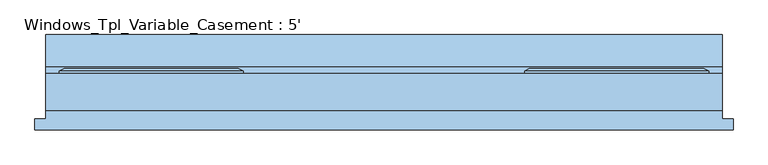
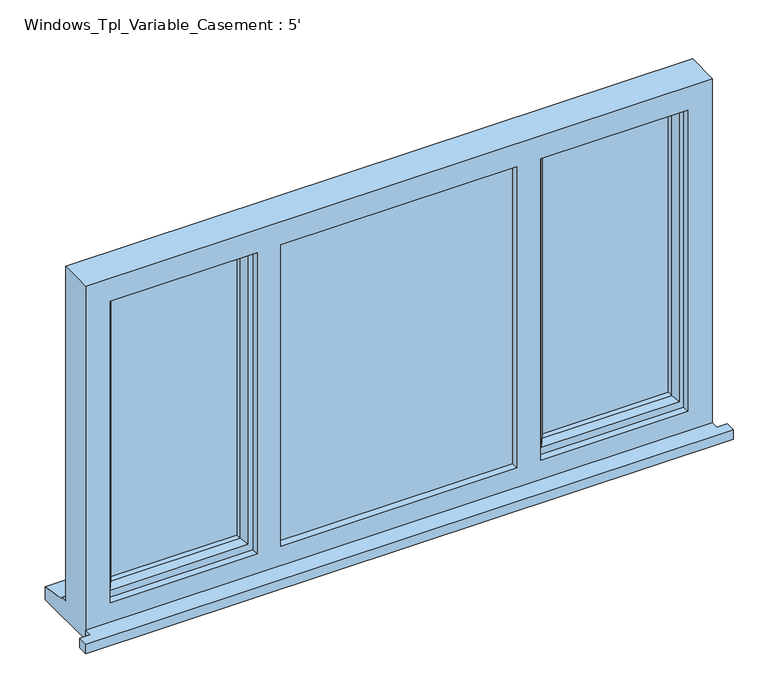
"""IFC4 building model written with IfcOpenShell, lengths in millimetres: window geometry, Windows_Tpl_Variable_Casement : 5'."""

from ifc_helpers import new_model, si_unit, frame, origin, place, context, project, spatial, polyline, outline, extrude, faceted_brep, source, transform, mapped, element, save


def windows_tpl_variable_casement_5_ffad3fa3(model_context):
    return source(origin(), model_context, "Body", "SolidModel", [
        extrude(outline(polyline([(-1234.0, -92.7434322), (-1234.0, -67.7434322), (-1209.0, -67.7434322), (-1209.0, -48.3434322), (315.0, -48.3434322), (315.0, -67.7434322), (340.0, -67.7434322), (340.0, -92.7434322), (-1234.0, -92.7434322)])), frame((0.0, 0.0, 1200.0), z_axis=(0.0, 0.0, 1.0), x_axis=(1.0, 0.0, 0.0)), (0.0, 0.0, 1.0), 25.0),
        faceted_brep([(-130.0, 34.6565678, 2080.0), (-130.0, 40.4300705, 2080.0), (-130.0, 40.4300705, 1253.0), (-130.0, 34.6565678, 1253.0), (-120.0, -30.3434322, 2070.0), (-120.0, 34.6565678, 2070.0), (-120.0, 34.6565678, 1263.0), (-120.0, -30.3434322, 1263.0), (-80.0, -15.8505323, 2030.0), (-90.1480377, -30.3434322, 2040.1480377), (-90.1480377, -30.3434322, 1292.8519623), (-80.0, -15.8505323, 1303.0), (-80.0, -1.3434322, 2030.0), (-80.0, -1.3434322, 1303.0), (-90.0, 22.6565678, 2040.0), (-90.0, -1.3434322, 2040.0), (-90.0, -1.3434322, 1293.0), (-90.0, 22.6565678, 1293.0), (-80.0, 40.4300705, 2030.0), (-80.0, 22.6565678, 2030.0), (-80.0, 22.6565678, 1303.0), (-80.0, 40.4300705, 1303.0), (-97.4457548, 46.2035732, 2047.4457548), (-97.4457548, 46.2035732, 1285.5542452), (-119.2153903, 46.2035732, 2069.2153903), (-119.2153903, 46.2035732, 1263.7846097), (285.0, 40.4300705, 1253.0), (285.0, 34.6565678, 1253.0), (275.0, 34.6565678, 1263.0), (275.0, -30.3434322, 1263.0), (245.1480377, -30.3434322, 1292.8519623), (235.0, -15.8505323, 1303.0), (235.0, -1.3434322, 1303.0), (245.0, -1.3434322, 1293.0), (245.0, 22.6565678, 1293.0), (235.0, 22.6565678, 1303.0), (235.0, 40.4300705, 1303.0), (252.4457548, 46.2035732, 1285.5542452), (274.2153903, 46.2035732, 1263.7846097), (285.0, 40.4300705, 2080.0), (285.0, 34.6565678, 2080.0), (275.0, 34.6565678, 2070.0), (275.0, -30.3434322, 2070.0), (245.1480377, -30.3434322, 2040.1480377), (235.0, -15.8505323, 2030.0), (235.0, -1.3434322, 2030.0), (245.0, -1.3434322, 2040.0), (245.0, 22.6565678, 2040.0), (235.0, 22.6565678, 2030.0), (235.0, 40.4300705, 2030.0), (252.4457548, 46.2035732, 2047.4457548), (274.2153903, 46.2035732, 2069.2153903)], [[[0, 1, 2, 3]], [[4, 5, 6, 7]], [[8, 9, 10, 11]], [[12, 8, 11, 13]], [[14, 15, 16, 17]], [[18, 19, 20, 21]], [[22, 18, 21, 23]], [[1, 24, 25, 2]], [[3, 2, 26, 27]], [[7, 6, 28, 29]], [[11, 10, 30, 31]], [[13, 11, 31, 32]], [[17, 16, 33, 34]], [[21, 20, 35, 36]], [[23, 21, 36, 37]], [[2, 25, 38, 26]], [[27, 26, 39, 40]], [[29, 28, 41, 42]], [[31, 30, 43, 44]], [[32, 31, 44, 45]], [[34, 33, 46, 47]], [[36, 35, 48, 49]], [[37, 36, 49, 50]], [[26, 38, 51, 39]], [[40, 39, 1, 0]], [[3, 27, 40, 0], [5, 41, 28, 6]], [[42, 41, 5, 4]], [[7, 29, 42, 4], [9, 43, 30, 10]], [[44, 43, 9, 8]], [[45, 44, 8, 12]], [[15, 46, 33, 16], [13, 32, 45, 12]], [[47, 46, 15, 14]], [[17, 34, 47, 14], [19, 48, 35, 20]], [[49, 48, 19, 18]], [[50, 49, 18, 22]], [[24, 51, 38, 25], [23, 37, 50, 22]], [[39, 51, 24, 1]]]),
        faceted_brep([(-764.0, 34.6565678, 2080.0), (-764.0, 40.4300705, 2080.0), (-1179.0, 40.4300705, 2080.0), (-1179.0, 34.6565678, 2080.0), (-774.0, -30.3434322, 2070.0), (-774.0, 34.6565678, 2070.0), (-1169.0, 34.6565678, 2070.0), (-1169.0, -30.3434322, 2070.0), (-814.0, -15.8505323, 2030.0), (-803.8519623, -30.3434322, 2040.1480377), (-1139.1480377, -30.3434322, 2040.1480377), (-1129.0, -15.8505323, 2030.0), (-814.0, -1.3434322, 2030.0), (-1129.0, -1.3434322, 2030.0), (-804.0, 22.6565678, 2040.0), (-804.0, -1.3434322, 2040.0), (-1139.0, -1.3434322, 2040.0), (-1139.0, 22.6565678, 2040.0), (-814.0, 40.4300705, 2030.0), (-814.0, 22.6565678, 2030.0), (-1129.0, 22.6565678, 2030.0), (-1129.0, 40.4300705, 2030.0), (-795.1854344, 46.2035732, 2048.8145656), (-1147.8145656, 46.2035732, 2048.8145656), (-775.6307806, 46.2035732, 2068.3692194), (-1167.3692194, 46.2035732, 2068.3692194), (-1179.0, 40.4300705, 1253.0), (-1179.0, 34.6565678, 1253.0), (-1169.0, 34.6565678, 1263.0), (-1169.0, -30.3434322, 1263.0), (-1139.1480377, -30.3434322, 1292.8519623), (-1129.0, -15.8505323, 1303.0), (-1129.0, -1.3434322, 1303.0), (-1139.0, -1.3434322, 1293.0), (-1139.0, 22.6565678, 1293.0), (-1129.0, 22.6565678, 1303.0), (-1129.0, 40.4300705, 1303.0), (-1147.8145656, 46.2035732, 1284.1854344), (-1167.3692194, 46.2035732, 1264.6307806), (-764.0, 40.4300705, 1253.0), (-764.0, 34.6565678, 1253.0), (-774.0, 34.6565678, 1263.0), (-774.0, -30.3434322, 1263.0), (-803.8519623, -30.3434322, 1292.8519623), (-814.0, -15.8505323, 1303.0), (-814.0, -1.3434322, 1303.0), (-804.0, -1.3434322, 1293.0), (-804.0, 22.6565678, 1293.0), (-814.0, 22.6565678, 1303.0), (-814.0, 40.4300705, 1303.0), (-795.1854344, 46.2035732, 1284.1854344), (-775.6307806, 46.2035732, 1264.6307806)], [[[0, 1, 2, 3]], [[4, 5, 6, 7]], [[8, 9, 10, 11]], [[12, 8, 11, 13]], [[14, 15, 16, 17]], [[18, 19, 20, 21]], [[22, 18, 21, 23]], [[1, 24, 25, 2]], [[3, 2, 26, 27]], [[7, 6, 28, 29]], [[11, 10, 30, 31]], [[13, 11, 31, 32]], [[17, 16, 33, 34]], [[21, 20, 35, 36]], [[23, 21, 36, 37]], [[2, 25, 38, 26]], [[27, 26, 39, 40]], [[0, 3, 27, 40], [41, 28, 6, 5]], [[29, 28, 41, 42]], [[4, 7, 29, 42], [43, 30, 10, 9]], [[31, 30, 43, 44]], [[32, 31, 44, 45]], [[46, 33, 16, 15], [12, 13, 32, 45]], [[34, 33, 46, 47]], [[14, 17, 34, 47], [48, 35, 20, 19]], [[36, 35, 48, 49]], [[37, 36, 49, 50]], [[51, 38, 25, 24], [22, 23, 37, 50]], [[26, 38, 51, 39]], [[40, 39, 1, 0]], [[42, 41, 5, 4]], [[44, 43, 9, 8]], [[45, 44, 8, 12]], [[47, 46, 15, 14]], [[49, 48, 19, 18]], [[50, 49, 18, 22]], [[39, 51, 24, 1]]]),
        faceted_brep([(315.0, -48.3434322, 2110.0), (-1209.0, -48.3434322, 2110.0), (-1209.0, -48.3434322, 1200.0), (315.0, -48.3434322, 1200.0), (255.0, -48.3434322, 2050.0), (255.0, -48.3434322, 1275.0), (-102.0, -48.3434322, 1275.0), (-102.0, -48.3434322, 2050.0), (-792.0, -48.3434322, 2050.0), (-792.0, -48.3434322, 1275.0), (-1149.0, -48.3434322, 1275.0), (-1149.0, -48.3434322, 2050.0), (-160.0, -48.3434322, 2050.0), (-160.0, -48.3434322, 1275.0), (-734.0, -48.3434322, 1275.0), (-734.0, -48.3434322, 2050.0), (-1209.0, 34.6565678, 2110.0), (-1209.0, 34.6565678, 1251.0), (-1209.0, 49.6565678, 1249.68767), (-1209.0, 49.6565678, 1244.7449676), (-1209.0, 122.1565678, 1233.8088847), (-1209.0, 122.1565678, 1200.0), (315.0, 34.6565678, 2110.0), (315.0, 34.6565678, 1251.0), (-1169.0, 34.6565678, 2070.0), (-1169.0, 34.6565678, 1263.0), (-774.0, 34.6565678, 1263.0), (-774.0, 34.6565678, 2070.0), (-120.0, 34.6565678, 2070.0), (-120.0, 34.6565678, 1263.0), (275.0, 34.6565678, 1263.0), (275.0, 34.6565678, 2070.0), (-734.0, 34.6565678, 2070.0), (-734.0, 34.6565678, 1263.0), (-160.0, 34.6565678, 1263.0), (-160.0, 34.6565678, 2070.0), (-1169.0, -30.3434322, 2070.0), (-1169.0, -30.3434322, 1263.0), (-744.0, -30.3434322, 2070.0), (-150.0, -30.3434322, 2070.0), (-150.0, -30.3434322, 1263.0), (-744.0, -30.3434322, 1263.0), (-160.0, -30.3434322, 2050.0), (-734.0, -30.3434322, 2050.0), (-734.0, -30.3434322, 1275.0), (-160.0, -30.3434322, 1275.0), (-120.0, -30.3434322, 2070.0), (275.0, -30.3434322, 2070.0), (275.0, -30.3434322, 1263.0), (-120.0, -30.3434322, 1263.0), (255.0, -30.3434322, 2050.0), (-102.0, -30.3434322, 2050.0), (-102.0, -30.3434322, 1275.0), (255.0, -30.3434322, 1275.0), (-774.0, -30.3434322, 2070.0), (-774.0, -30.3434322, 1263.0), (-792.0, -30.3434322, 2050.0), (-1149.0, -30.3434322, 2050.0), (-1149.0, -30.3434322, 1275.0), (-792.0, -30.3434322, 1275.0), (-734.0, -6.3434322, 2070.0), (-160.0, -6.3434322, 2070.0), (-150.0, -6.3434322, 2070.0), (-744.0, -6.3434322, 2070.0), (315.0, 122.1565678, 1200.0), (315.0, 122.1565678, 1233.8088847), (315.0, 49.6565678, 1244.7449676), (315.0, 49.6565678, 1249.68767), (-734.0, -6.3434322, 1263.0), (-744.0, -6.3434322, 1263.0), (-150.0, -6.3434322, 1263.0), (-160.0, -6.3434322, 1263.0)], [[[0, 1, 2, 3], [4, 5, 6, 7], [8, 9, 10, 11], [12, 13, 14, 15]], [[2, 1, 16, 17, 18, 19, 20, 21]], [[17, 16, 22, 23], [24, 25, 26, 27], [28, 29, 30, 31], [32, 33, 34, 35]], [[25, 24, 36, 37]], [[38, 39, 40, 41], [42, 43, 44, 45]], [[46, 47, 48, 49], [50, 51, 52, 53]], [[36, 54, 55, 37], [56, 57, 58, 59]], [[57, 11, 10, 58]], [[1, 0, 22, 16]], [[36, 24, 27, 54]], [[31, 47, 46, 28]], [[60, 32, 35, 61, 62, 39, 38, 63]], [[11, 57, 56, 8]], [[50, 4, 7, 51]], [[15, 43, 42, 12]], [[23, 22, 0, 3, 64, 65, 66, 67]], [[31, 30, 48, 47]], [[4, 50, 53, 5]], [[43, 15, 14, 44]], [[8, 56, 59, 9]], [[27, 26, 55, 54]], [[33, 32, 60, 68]], [[68, 60, 63, 69]], [[69, 63, 38, 41]], [[62, 70, 40, 39]], [[70, 62, 61, 71]], [[71, 61, 35, 34]], [[29, 28, 46, 49]], [[51, 7, 6, 52]], [[12, 42, 45, 13]], [[64, 3, 2, 21]], [[65, 64, 21, 20]], [[66, 65, 20, 19]], [[67, 66, 19, 18]], [[23, 67, 18, 17]], [[26, 25, 37, 55]], [[30, 29, 49, 48]], [[41, 40, 70, 71, 34, 33, 68, 69]], [[6, 5, 53, 52]], [[59, 58, 10, 9]], [[45, 44, 14, 13]]]),
        extrude(outline(polyline([(-804.0, -1.3434322), (-1139.0, -1.3434322), (-1139.0, 22.6565678), (-804.0, 22.6565678), (-804.0, -1.3434322)])), frame((0.0, 0.0, 1293.0), z_axis=(0.0, 0.0, 1.0), x_axis=(1.0, 0.0, 0.0)), (0.0, 0.0, 1.0), 747.0),
        extrude(outline(polyline([(-744.0, -6.3434322), (-150.0, -6.3434322), (-150.0, -30.3434322), (-744.0, -30.3434322), (-744.0, -6.3434322)])), frame((0.0, 0.0, 1263.0), z_axis=(0.0, 0.0, 1.0), x_axis=(1.0, 0.0, 0.0)), (0.0, 0.0, 1.0), 807.0),
        extrude(outline(polyline([(245.0, -1.3434322), (-90.0, -1.3434322), (-90.0, 22.6565678), (245.0, 22.6565678), (245.0, -1.3434322)])), frame((0.0, 0.0, 1293.0), z_axis=(0.0, 0.0, 1.0), x_axis=(1.0, 0.0, 0.0)), (0.0, 0.0, 1.0), 747.0),
    ])


if __name__ == "__main__":
    model = new_model("IFC4")
    model_context = context("Model", 3, world=origin())
    ifc_project = project(units=[si_unit("LENGTHUNIT", "METRE", prefix="MILLI")], contexts=[model_context])
    site = spatial("IfcSite", under=ifc_project)
    building = spatial("IfcBuilding", under=site)
    placement = place(None, origin())
    windows_tpl_variable_casement_5_shape = windows_tpl_variable_casement_5_ffad3fa3(model_context)
    element("IfcWindow", 1, ObjectType="Windows_Tpl_Variable_Casement : 5'", at=placement, inside=building, context=model_context, shape_type="MappedRepresentation", body=[
        mapped(windows_tpl_variable_casement_5_shape, transform((0.0, 0.0, 0.0), x_axis=(1.0, 0.0, 0.0), y_axis=(0.0, 1.0, 0.0), z_axis=(0.0, 0.0, 1.0))),
    ])
    save(model, "model.ifc")

# Revit data of these elements
# Type "Windows_Tpl_Variable_Casement : 5'"
#   Type Mark = "83"
#   Operation = "TriplePanelVertical"
#   Construction Type Id = "GSP4R"
#   Manufacturer = "Revit"
#   Keynote = "L10"
#   Analytic Construction = "1/8 in Pilkington single glazing"
#   Wrap Layers (Int) from Ext = 177.5 mm
#   Wrap Layers (Ext) from Ext = 102.5 mm
#   Window Board Projection = 25 mm
#   Window Board Extension = 25 mm
#   Visual Light Transmittance = 0.9
#   Solar Heat Gain Coefficient = 0.78
#   Rough Width = 1524 mm
#   Rough Height = 910 mm
#   Height = 910 mm
#   Width = 1524 mm
#   Heat Transfer Coefficient (U) = 3.6886 W/(m²·K)
#   Glazing Thickness = 24 mm
#   FrameOffset - External = 50 mm
#   Frame Depth = 65 mm
#   Default Head Height = 2110 mm
#   Cill Depth = 87.5 mm
#   Cavity Closer Width = 50 mm
#   Cavity Closer Offset from Ext = 102.5 mm
#   Cavity Closer Depth = 85 mm
#   Casement Width = 450 mm
#   Vis - Cavity Closers = yes
#   Define Thermal Properties by = 1
#   Material Trim = Window Frame
#   Material Glass = Glass
#   Material Frame = Window Frame
#   Wall Closure = (empty or 0)
# Element 1 (IfcWindow, "Windows_Tpl_Variable_Casement : 5'")
#   Materials on its faces: "Window Frame", "Glass"
# Materials
#   "Window Frame": colour RGB 249 249 249, transparency 0, Keynote = "L10", Cost = 0
#   "Glass": class "Glass", colour RGB 0 128 192, transparency 0.9, Description = "Soda Lime Glass", Cost = 0
